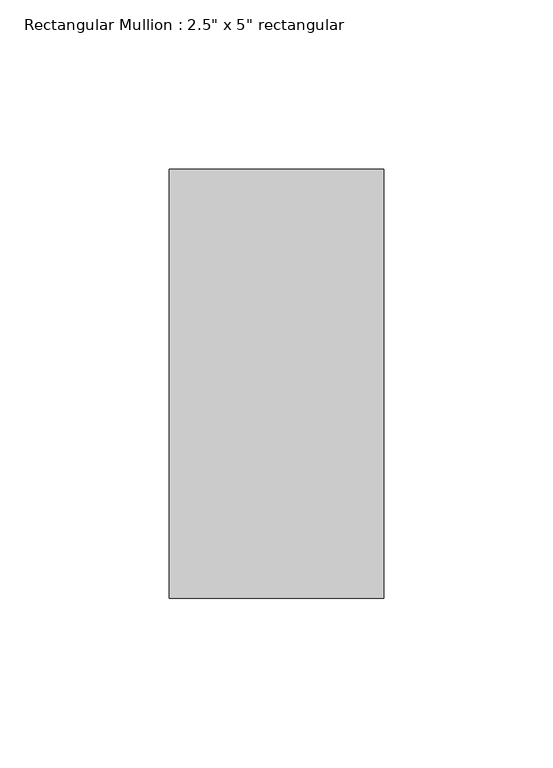
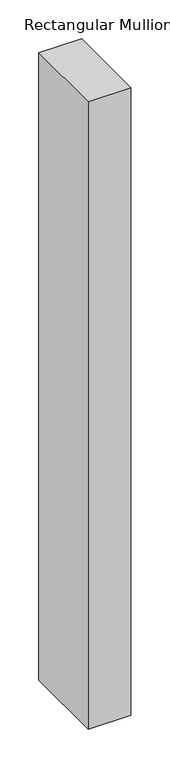
"""IFC4 building model written with IfcOpenShell, lengths in millimetres: member geometry."""

from ifc_helpers import new_model, si_unit, frame, origin, place, context, project, spatial, polyline, outline, extrude, source, transform, mapped, element, save


def member_f2556e69(model_context):
    return source(origin(), model_context, "Body", "SweptSolid", [
        extrude(outline(polyline([(0.0, 63.5), (0.0, -63.5), (-63.5, -63.5), (-63.5, 63.5), (0.0, 63.5)])), frame((0.0, 0.0, -986.3666665), z_axis=(0.0, 0.0, 1.0), x_axis=(1.0, 0.0, 0.0)), (0.0, 0.0, 1.0), 986.3666665),
    ])


if __name__ == "__main__":
    model = new_model("IFC4")
    model_context = context("Model", 3, world=origin())
    ifc_project = project(units=[si_unit("LENGTHUNIT", "METRE", prefix="MILLI")], contexts=[model_context])
    site = spatial("IfcSite", under=ifc_project)
    building = spatial("IfcBuilding", under=site)
    placement = place(None, origin())
    member_shape = member_f2556e69(model_context)
    element("IfcMember", 1, ObjectType="Rectangular Mullion : 2.5\" x 5\" rectangular", at=placement, inside=building, context=model_context, shape_type="MappedRepresentation", body=[
        mapped(member_shape, transform((0.0, 0.0, 0.0), x_axis=(1.0, 0.0, 0.0), y_axis=(0.0, 1.0, 0.0), z_axis=(0.0, 0.0, 1.0))),
    ])
    save(model, "model.ifc")

# Revit data of these elements
# Type "Rectangular Mullion : 2.5\" x 5\" rectangular"
#   built-in parameter 1007304 = 0.416667 (stored number, unit not read)
#   built-in parameter 1007301 = 0.104167 (stored number, unit not read)
#   built-in parameter 1007300 = 0.104167 (stored number, unit not read)
# Element 1 (IfcMember, "Rectangular Mullion : 2.5\" x 5\" rectangular")
#   Materials on its faces: "Aluminum"
# Materials
#   "Aluminum": class "Metal", colour RGB 247 247 247, transparency 0, Description = "Aluminum 6061", Cost = 0
